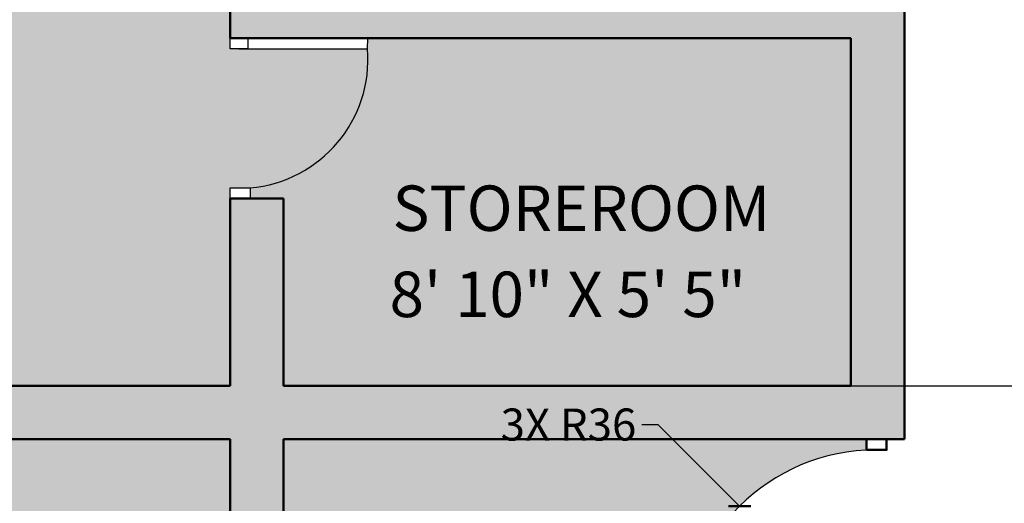
# Model space of a CAD drawing. Units: inches. Extents: x 925 to 2834, y 111 to 1355.
# Tile 18 of 25: x 1553 to 1737, y 882 to 972. Entities that reach past the tile are written whole.
import ezdxf

# ---------------------------------------------------------------- set-up
doc = ezdxf.new("R2010")
doc.units = ezdxf.units.IN
doc.header["$MEASUREMENT"] = 0
for name, color, linetype, lineweight in [('A-ANNO-DIMS', 2, 'Continuous', 18), ('A-AREA-IDEN', 7, 'Continuous', 18), ('A-DOOR', 2, 'Continuous', 25), ('A-FLOR-PATT', 252, 'Continuous', 13), ('A-WALL', 7, 'Continuous', 50)]:
    doc.layers.add(name, color=color, linetype=linetype, lineweight=lineweight)
doc.styles.get("Standard").update_dxf_attribs({"font": 'arial.ttf'})
doc.dimstyles.get("Standard").update_dxf_attribs({"dimtxt": 6, "dimasz": 3, "dimexe": 0.18, "dimexo": 0.0625, "dimgap": 0.09, "dimtad": 0, "dimtih": 1, "dimtoh": 1, "dimdec": 1, "dimzin": 0, "dimdsep": 46, "dimlunit": 3, "dimtxsty": 'Standard', "dimblk": 'ARCHTICK', "dimcen": 0.09, "dimadec": 0, "dimazin": 0, "dimtfac": 1, "dimtdec": 1, "dimtofl": 0, "dimtmove": 0, "dimatfit": 3, "dimfxl": 1, "dimtolj": 1, "dimtzin": 0, "dimarcsym": 0})

# ---------------------------------------------------------------- blocks, each defined once
blk = doc.blocks.new('_ArchTick')
at = {"color": 0, "linetype": 'ByBlock', "const_width": 0.15}
blk.add_lwpolyline([(-0.5, -0.5), (0.5, 0.5)], dxfattribs=at)
blk = doc.blocks.new('*D47')
at = {"layer": 'A-ANNO-DIMS', "color": 0, "lineweight": -2, "transparency": 16777216}
for p, q in [((1708.78, 903.59), (1988.62, 903.59)), ((1988.44, 903.59), (1988.44, 869.23)), ((1988.44, 828.59), (1988.44, 862.95)), ((1708.78, 828.59), (1988.62, 828.59))]:
    blk.add_line(p, q, dxfattribs=at)
at = {"layer": 'Defpoints', "color": 0, "transparency": 16777216}
for p in [(1708.71, 903.59), (1988.44, 903.59), (1708.71, 828.59)]:
    blk.add_point(p, dxfattribs=at)
at = {"layer": 'A-ANNO-DIMS', "color": 0, "lineweight": -2, "transparency": 16777216, "xscale": 3, "yscale": 3, "zscale": 3}
for p, rotation in [((1988.44, 903.59), 90), ((1988.44, 828.59), 270)]:
    blk.add_blockref('_ArchTick', p, dxfattribs=dict(at, rotation=rotation))
at = {"layer": 'A-ANNO-DIMS', "color": 0, "transparency": 16777216, "insert": (1988.44, 866.09), "char_height": 6, "attachment_point": 5}
blk.add_mtext('\\A1;75', dxfattribs=at)
blk = doc.blocks.new('*D48')
at = {"layer": 'A-ANNO-DIMS', "color": 0, "lineweight": -2, "transparency": 16777216}
for p, q in [((1708.78, 975.59), (1988.62, 975.59)), ((1988.44, 975.59), (1988.44, 942.69)), ((1988.44, 903.59), (1988.44, 936.49)), ((1708.78, 903.59), (1988.62, 903.59))]:
    blk.add_line(p, q, dxfattribs=at)
at = {"layer": 'Defpoints', "color": 0, "transparency": 16777216}
for p in [(1708.71, 975.59), (1988.44, 975.59), (1708.71, 903.59)]:
    blk.add_point(p, dxfattribs=at)
at = {"layer": 'A-ANNO-DIMS', "color": 0, "lineweight": -2, "transparency": 16777216, "xscale": 3, "yscale": 3, "zscale": 3}
for p, rotation in [((1988.44, 975.59), 90), ((1988.44, 903.59), 270)]:
    blk.add_blockref('_ArchTick', p, dxfattribs=dict(at, rotation=rotation))
at = {"layer": 'A-ANNO-DIMS', "color": 0, "transparency": 16777216, "insert": (1988.44, 939.59), "char_height": 6, "attachment_point": 5}
blk.add_mtext('\\A1;72', dxfattribs=at)
blk = doc.blocks.new('*D81')
at = {"layer": 'A-ANNO-DIMS', "color": 0, "lineweight": -2, "transparency": 16777216}
for p, q in [((1669.64, 896.32), (1672.64, 896.32)), ((1672.64, 896.32), (1687.92, 881.04)), ((1713.28, 855.59), (1713.46, 855.59)), ((1713.37, 855.5), (1713.37, 855.68))]:
    blk.add_line(p, q, dxfattribs=at)
at = {"layer": 'Defpoints', "color": 0, "transparency": 16777216}
for p in [(1687.92, 881.04), (1713.37, 855.59)]:
    blk.add_point(p, dxfattribs=at)
at = {"layer": 'A-ANNO-DIMS', "color": 0, "lineweight": -2, "transparency": 16777216, "xscale": 3, "yscale": 3, "zscale": 3, "rotation": 315.0000844046568}
blk.add_blockref('_ArchTick', (1687.92, 881.04), dxfattribs=at)
at = {"layer": 'A-ANNO-DIMS', "color": 0, "transparency": 16777216, "insert": (1655.94, 896.32), "char_height": 6, "attachment_point": 5}
blk.add_mtext('\\A1;3X R36', dxfattribs=at)

msp = doc.modelspace()

# ---------------------------------------------------------------- hatches: boundary and pattern name
at = {"layer": 'A-FLOR-PATT', "transparency": 33554605}
h = msp.add_hatch(color=256, dxfattribs=at)
h.dxf.hatch_style = 1
h.paths.add_polyline_path([(1931.688, 1294.5638), (991.7375, 1294.5638), (991.7375, 172.1134), (1931.688, 172.1134)])
h.paths.add_polyline_path([(1910.7128, 1273.5886), (1910.7128, 193.0886), (1012.7128, 193.0886), (1012.7128, 1273.5886)], flags=16)
h.paths.add_polyline_path([(1850.7128, 1213.5886), (1850.7128, 253.0886), (1072.7128, 253.0886), (1072.7128, 1213.5886)], flags=0)
h.paths.add_polyline_path([(1838.7128, 1201.5886), (1838.7128, 265.0886), (1084.7128, 265.0886), (1084.7128, 530.5886), (1084.7128, 1201.5886)], flags=0)
h.paths.add_polyline_path([(1547.6758, 1155.7396), (1547.6758, 1119.115), (1513.0687, 1119.115), (1513.0687, 1155.7396)], flags=0)
h.paths.add_polyline_path([(1600.1067, 1154.9439), (1634.7139, 1154.9439), (1634.7139, 1119.115), (1600.1067, 1119.115)], flags=0)
h.paths.add_polyline_path([(1505.2502, 1144.5358), (1505.2502, 1119.115), (1470.643, 1119.115), (1470.643, 1144.5358)], flags=0)
h.paths.add_polyline_path([(1559.1357, 1141.0962), (1593.7428, 1141.0962), (1593.7428, 1119.115), (1559.1357, 1119.115)], flags=0)
h.paths.add_polyline_path([(1462.8966, 1154.9439), (1462.8966, 1119.115), (1428.2895, 1119.115), (1428.2895, 1154.9439)], flags=0)
h.paths.add_polyline_path([(1642.4603, 1144.5358), (1677.0675, 1144.5358), (1677.0675, 1119.115), (1642.4603, 1119.115)], flags=0)
h.paths.add_polyline_path([(1422.3508, 1141.0962), (1422.3508, 1119.115), (1387.7436, 1119.115), (1387.7436, 1141.0962)], flags=0)
h.paths.add_polyline_path([(1684.8859, 1155.7396), (1719.4931, 1155.7396), (1719.4931, 1119.115), (1684.8859, 1119.115)], flags=0)
h.paths.add_polyline_path([(1718.7128, 1081.5886), (1718.7128, 1050.1249), (1715.7128, 1050.1249), (1715.7128, 1026.1249), (1715.7128, 1002.1249), (1718.7128, 1002.1249), (1730.7128, 1002.1249), (1730.7128, 998.1249), (1730.7128, 990.1249), (1730.7128, 986.1249), (1718.7128, 986.1249), (1718.7128, 893.5886), (1715.3735, 893.5886), (1715.3735, 891.5886), (1713.3735, 891.5886, 0.41421356), (1677.3735, 855.5886), (1713.3735, 855.5886), (1713.3735, 853.5886), (1715.3735, 853.5886), (1715.3735, 851.5886), (1718.7128, 851.5886), (1718.7128, 821.5865), (1734.4655, 821.5865), (1734.3735, 819.5886, -0.41421356), (1712.4415, 793.5886), (1712.4415, 791.5886), (1718.7128, 791.5886), (1718.7128, 717.5886), (1718.7128, 669.5886), (1732.7128, 669.5886), (1732.7128, 665.5886), (1732.7128, 641.5886), (1732.7128, 634.5886), (1732.7128, 610.5886), (1732.7128, 603.5886), (1718.7128, 603.5886), (1718.7128, 385.0886), (1434.2128, 385.0886), (1434.2128, 530.5886), (1410.2128, 530.5886), (1408.2128, 530.5886), (1408.2128, 532.5886, 0.41421356), (1372.2128, 568.5886), (1372.2128, 532.5886), (1370.2128, 532.5886), (1370.2128, 530.5886), (1368.2128, 530.5886), (1282.2128, 530.5886), (1210.2128, 530.5886), (1200.2128, 530.5886), (1200.2128, 542.1915), (1183.2307, 542.1915), (1183.2307, 546.1915), (1200.2128, 546.1915), (1200.2128, 572.1915), (1183.2307, 572.1915), (1183.2307, 576.1915), (1200.2128, 576.1915), (1200.2128, 727.5886), (1210.2128, 727.5886), (1234.2128, 727.5886), (1259.7128, 727.5886), (1259.7128, 775.5886), (1259.7128, 799.5886), (1259.7128, 847.5886), (1259.7128, 993.5872), (1259.7128, 1065.5872), (1259.7128, 1071.5886), (1219.6318, 1071.5886), (1219.6318, 1081.5886), (1084.7128, 1081.5886), (1084.7128, 1119.115), (1256.8974, 1119.115), (1256.8974, 1154.9439), (1291.5046, 1154.9439), (1291.5046, 1119.115), (1256.8974, 1119.115), (1256.6723, 1081.5886), (1293.7128, 1081.5886), (1341.7128, 1081.5886), (1341.7128, 1093.5886), (1347.7128, 1093.5886), (1371.7128, 1093.5886), (1377.7128, 1093.5886), (1377.7128, 1081.5886), (1668.7128, 1081.5886), (1668.7128, 1117.5886), (1675.7128, 1117.5886), (1711.7128, 1117.5886), (1718.7128, 1117.5886)], flags=0)
h.paths.add_polyline_path([(1376.2838, 1155.7396), (1376.2838, 1119.115), (1341.6766, 1119.115), (1341.6766, 1155.7396)], flags=0)
h.paths.add_polyline_path([(1341.7128, 1076.0886), (1293.7128, 1076.0886), (1293.7128, 1071.5886), (1269.7128, 1071.5886), (1269.7128, 1065.5872), (1266.7128, 1065.5872), (1266.7128, 1029.5872), (1265.7128, 1029.5872), (1265.7128, 993.5872), (1269.7128, 993.5872), (1269.7128, 903.5886), (1269.7128, 893.5886), (1269.7128, 847.5886), (1265.2128, 847.5886), (1265.2128, 799.5886), (1269.7128, 799.5886), (1269.7128, 775.5886), (1265.2128, 775.5886), (1265.2128, 727.5886), (1269.7128, 727.5886), (1444.2128, 727.5886), (1444.2128, 717.5886), (1234.2128, 717.5886), (1234.2128, 722.0886), (1210.2128, 722.0886), (1210.2128, 717.5886), (1210.2128, 540.5886), (1210.2128, 536.0886), (1282.2128, 536.0886), (1282.2128, 535.0886), (1210.2128, 535.0886), (1210.2128, 540.5886), (1210.2128, 717.5886), (1210.2128, 723.0886), (1234.2128, 723.0886), (1234.2128, 717.5886), (1444.2128, 717.5886), (1444.2128, 727.5886), (1269.7128, 727.5886), (1264.2128, 727.5886), (1264.2128, 775.5886), (1269.7128, 775.5886), (1269.7128, 799.5886), (1264.2128, 799.5886), (1264.2128, 847.5886), (1269.7128, 847.5886), (1269.7128, 893.5886), (1269.7128, 903.5886), (1269.7128, 993.5872), (1264.7128, 993.5872), (1264.7128, 1029.5872), (1265.7128, 1029.5872), (1265.7128, 1065.5872), (1269.7128, 1065.5872), (1269.7128, 1071.5886), (1293.7128, 1071.5886), (1293.7128, 1077.0886), (1341.7128, 1077.0886)], flags=0)
h.paths.add_polyline_path([(1730.9529, 1141.0962), (1765.5601, 1141.0962), (1765.5601, 1119.115), (1730.9529, 1119.115)], flags=0)
h.paths.add_polyline_path([(1333.8582, 1144.5358), (1333.8582, 1119.115), (1299.251, 1119.115), (1299.251, 1144.5358)], flags=0)
h.paths.add_polyline_path([(1592.7128, 968.5886), (1596.0342, 968.5886), (1602.7128, 968.5886), (1708.7128, 968.5886), (1708.7128, 903.5886), (1602.7128, 903.5886), (1602.7128, 938.5886), (1592.7128, 938.5886), (1592.7128, 903.5886), (1451.7128, 903.5886), (1451.7128, 893.5886), (1511.7128, 893.5886), (1511.7128, 881.5886), (1515.2128, 881.5886), (1518.7128, 881.5886), (1518.7128, 893.5886), (1592.7128, 893.5886), (1592.7128, 799.5886), (1518.7128, 799.5886), (1518.7128, 857.5886), (1511.7128, 857.5886), (1511.7128, 799.5886), (1511.7128, 772.0886), (1521.7128, 772.0886), (1521.7128, 792.5886), (1592.7128, 792.5886), (1592.7128, 727.5886), (1521.7128, 727.5886), (1521.7128, 748.0886), (1511.7128, 748.0886), (1511.7128, 717.5886), (1708.7128, 717.5886), (1714.2128, 717.5886), (1714.2128, 669.5886), (1708.7128, 669.5886), (1708.7128, 641.5886), (1492.2128, 641.5886), (1492.2128, 631.5886), (1621.2128, 631.5886), (1621.2128, 443.0886), (1625.7128, 443.0886), (1625.7128, 503.0886), (1625.7128, 507.5886), (1625.7128, 631.5886), (1708.7128, 631.5886), (1708.7128, 507.5886), (1655.7128, 507.5886), (1655.7128, 503.0886), (1708.7128, 503.0886), (1708.7128, 395.0886), (1625.7128, 395.0886), (1625.7128, 419.0886), (1621.2128, 419.0886), (1621.2128, 395.0886), (1482.2128, 395.0886), (1482.2128, 385.0886), (1434.2128, 385.0886), (1434.2128, 433.0886), (1444.2128, 433.0886), (1444.2128, 631.5886), (1450.2128, 631.5886), (1450.2128, 634.91), (1452.2128, 634.91), (1452.2128, 669.5886), (1454.2128, 669.5886, -0.40021217), (1490.1712, 635.3173), (1492.2128, 635.3173), (1492.2128, 641.5886), (1564.7128, 641.5886), (1564.7128, 677.5886), (1672.7128, 677.5886), (1672.7128, 681.5886), (1564.7128, 681.5886), (1564.7128, 717.5886), (1511.7128, 717.5886), (1511.7128, 748.0886), (1511.7128, 772.0886), (1511.7128, 799.5886), (1511.7128, 857.5886), (1511.8913, 857.5886), (1511.8913, 859.5886), (1515.6201, 859.5886, 0.41421356), (1537.552, 879.5886), (1513.552, 879.5886), (1511.8913, 879.5886), (1511.8913, 881.5886), (1511.7128, 881.5886), (1511.7128, 893.5886), (1451.7128, 893.5886), (1451.7128, 903.5886), (1592.7128, 903.5886), (1592.7128, 938.5886), (1592.7128, 940.5886), (1596.4415, 940.5886, 0.41421356), (1618.3735, 966.5886), (1594.3735, 966.5886), (1592.7128, 966.5886)], flags=0)
h.paths.add_polyline_path([(1377.7128, 903.5886), (1377.7128, 893.5886), (1305.7128, 893.5886), (1305.7128, 903.5886)], flags=0)
h.paths.add_polyline_path([(1708.7128, 821.5886), (1712.0342, 821.5886), (1712.0342, 819.5886), (1710.3735, 819.5886), (1708.7128, 819.5886)], flags=0)
h.paths.add_polyline_path([(1576.7128, 695.1992), (1575.5896, 693.6649), (1575.9687, 694.6994), (1575.4438, 695.1992), (1575.9687, 695.699), (1575.5896, 696.7335)], flags=0)
h.paths.add_polyline_path([(1565.9817, 662.3134), (1565.4568, 661.8136), (1565.8359, 660.7791), (1564.7128, 662.3134), (1565.8359, 663.8477), (1565.4568, 662.8132)], flags=0)
h.paths.add_polyline_path([(1444.2128, 433.0886), (1444.2128, 395.0886), (1482.2128, 395.0886), (1482.2128, 389.0886), (1438.2128, 389.0886), (1438.2128, 391.8608), (1438.2128, 433.0886)], flags=0)
h.paths.add_polyline_path([(1410.2128, 506.5886), (1410.2128, 289.0886), (1108.7128, 289.0886), (1108.7128, 506.5886)], flags=0)
h.paths.add_polyline_path([(1612.3153, 838.3016), (1680.4151, 838.3016), (1680.4151, 851.3131), (1612.3153, 851.3131)], flags=8)
h.paths.add_polyline_path([(1208.3174, 395.0436), (1282.1017, 395.0436), (1282.1017, 408.0552), (1208.3174, 408.0552)], flags=8)
h.paths.add_polyline_path([(1291.8049, 598.7427), (1369.8017, 598.7427), (1369.8017, 611.7542), (1291.8049, 611.7542)], flags=8)
h.paths.add_polyline_path([(1119.679, 917.3022), (1191.0817, 917.3022), (1191.0817, 930.3137), (1119.679, 930.3137)], flags=8)
h.paths.add_polyline_path([(1332.2261, 815.9808), (1410.2258, 815.9808), (1410.2258, 829.001), (1332.2261, 829.001)], flags=8)
h.paths.add_polyline_path([(1390.9013, 955.8158), (1475.4981, 955.8158), (1475.4981, 968.8273), (1390.9013, 968.8273)], flags=8)
h.paths.add_polyline_path([(1620.3436, 998.9325), (1688.4434, 998.9325), (1688.4434, 1011.944), (1620.3436, 1011.944)], flags=8)
h.paths.add_polyline_path([(1620.3436, 914.1039), (1691.7405, 914.1039), (1691.7405, 927.1155), (1620.3436, 927.1155)], flags=8)
h.paths.add_polyline_path([(1521.4542, 816.005), (1589.5569, 816.005), (1589.5569, 829.0253), (1521.4542, 829.0253)], flags=8)
h.paths.add_polyline_path([(1528.524, 740.3497), (1602.3082, 740.3497), (1602.3082, 753.3613), (1528.524, 753.3613)], flags=8)
h.paths.add_polyline_path([(1627.6094, 762.6128), (1702.3091, 762.6128), (1702.3091, 775.6244), (1627.6094, 775.6244)], flags=8)
h.paths.add_polyline_path([(1610.5442, 657.2751), (1684.3284, 657.2751), (1684.3284, 670.2867), (1610.5442, 670.2867)], flags=8)
h.paths.add_polyline_path([(1636.6983, 519.472), (1711.3981, 519.472), (1711.3981, 532.4835), (1636.6983, 532.4835)], flags=8)
h.paths.add_polyline_path([(1616.8577, 424.8539), (1694.8545, 424.8539), (1694.8545, 437.8654), (1616.8577, 437.8654)], flags=8)
h.paths.add_polyline_path([(1506.1456, 460.8838), (1579.9299, 460.8838), (1579.9299, 473.8953), (1506.1456, 473.8953)], flags=8)
h.paths.add_polyline_path([(1624.6119, 784.6011), (1696.9185, 784.6011), (1696.9185, 797.7864), (1624.6119, 797.7864)], flags=8)
h.paths.add_polyline_path([(1606.3732, 854.2194), (1683.3039, 854.2194), (1683.3039, 867.4048), (1606.3732, 867.4048)], flags=8)
h.paths.add_polyline_path([(1127.8008, 940.3581), (1165.1637, 940.3581), (1165.1637, 953.5348), (1127.8008, 953.5348)], flags=8)
h.paths.add_polyline_path([(1620.8657, 1019.4968), (1677.3447, 1019.4968), (1677.3447, 1032.6735), (1620.8657, 1032.6735)], flags=8)
h.paths.add_polyline_path([(1620.8643, 930.1821), (1703.0564, 930.1821), (1703.0564, 943.3675), (1620.8643, 943.3675)], flags=8)
h.paths.add_polyline_path([(1324.5702, 836.8338), (1408.0892, 836.8338), (1408.0892, 850.0191), (1324.5702, 850.0191)], flags=8)
h.paths.add_polyline_path([(1281.6584, 622.8885), (1383.6213, 622.8885), (1383.6213, 636.0739), (1281.6584, 636.0739)], flags=8)
h.paths.add_polyline_path([(1210.6721, 416.7893), (1269.1299, 416.7893), (1269.1299, 429.9747), (1210.6721, 429.9747)], flags=8)
h.paths.add_polyline_path([(1507.8264, 477.4836), (1586.7329, 477.4836), (1586.7329, 490.669), (1507.8264, 490.669)], flags=8)
h.paths.add_polyline_path([(1643.6238, 443.8135), (1696.6696, 443.8135), (1696.6696, 456.5643), (1643.6238, 456.5643)], flags=8)
h.paths.add_polyline_path([(1647.2466, 540.5638), (1693.1825, 540.5638), (1693.1825, 553.7491), (1647.2466, 553.7491)], flags=8)
h.paths.add_polyline_path([(1626.0633, 668.5064), (1673.3174, 668.5064), (1673.3174, 681.6831), (1626.0633, 681.6831)], flags=8)
h.paths.add_polyline_path([(1538.2915, 830.7872), (1567.5942, 830.7872), (1567.5942, 843.5293), (1538.2915, 843.5293)], flags=8)
h.paths.add_polyline_path([(1530.9338, 754.0477), (1559.576, 754.0477), (1559.576, 766.7898), (1530.9338, 766.7898)], flags=8)
h.paths.add_polyline_path([(1351.2461, 979.2309), (1513.8919, 979.2309), (1513.8919, 992.4076), (1351.2461, 992.4076)], flags=8)
at = {"layer": 'A-FLOR-PATT'}
h = msp.add_hatch(color=256, dxfattribs=at)
h.dxf.hatch_style = 1
h.paths.add_polyline_path([(1850.7128, 1213.5886), (1072.7128, 1213.5886), (1072.7128, 253.0886), (1850.7128, 253.0886)])
h.paths.add_polyline_path([(1084.7128, 1201.5886), (1838.7128, 1201.5886), (1838.7128, 265.0886), (1084.7128, 265.0886)], flags=16)
h.paths.add_polyline_path([(1183.2307, 576.1915), (1200.2128, 576.1915), (1200.2128, 727.5886), (1210.2128, 727.5886), (1234.2128, 727.5886), (1259.7128, 727.5886), (1259.7128, 775.5886), (1259.7128, 799.5886), (1259.7128, 847.5886), (1259.7128, 993.5872), (1259.7128, 1065.5872), (1259.7128, 1071.5886), (1219.6318, 1071.5886), (1219.6318, 1081.5886), (1293.7128, 1081.5886), (1341.7128, 1081.5886), (1341.7128, 1093.5886), (1347.7128, 1093.5886), (1347.7128, 1081.5886), (1371.7128, 1081.5886), (1371.7128, 1093.5886), (1377.7128, 1093.5886), (1377.7128, 1081.5886), (1668.7128, 1081.5886), (1668.7128, 1117.5886), (1675.7128, 1117.5886), (1675.7128, 1081.5886), (1711.7128, 1081.5886), (1711.7128, 1117.5886), (1718.7128, 1117.5886), (1718.7128, 1081.5886), (1718.7128, 1050.1249), (1715.7128, 1050.1249), (1715.7128, 1026.1249), (1715.7128, 1002.1249), (1718.7128, 1002.1249), (1730.7128, 1002.1249), (1730.7128, 998.1249), (1730.7128, 990.1249), (1730.7128, 986.1249), (1718.7128, 986.1249), (1718.7128, 893.5886), (1715.3735, 893.5886), (1715.3735, 891.5886), (1713.3735, 891.5886, 0.41421356), (1677.3735, 855.5886), (1713.3735, 855.5886), (1713.3735, 853.5886), (1715.3735, 853.5886), (1715.3735, 851.5886), (1718.7128, 851.5886), (1718.7128, 821.5865), (1734.4655, 821.5865), (1734.3735, 819.5886, -0.41421356), (1712.4415, 793.5886), (1712.4415, 791.5886), (1718.7128, 791.5886), (1718.7128, 717.5886), (1718.7128, 669.5886), (1732.7128, 669.5886), (1732.7128, 665.5886), (1732.7128, 641.5886), (1732.7128, 634.5886), (1732.7128, 610.5886), (1732.7128, 603.5886), (1718.7128, 603.5886), (1718.7128, 385.0886), (1434.2128, 385.0886), (1434.2128, 433.0886), (1434.2128, 530.5886), (1410.2128, 530.5886), (1408.2128, 530.5886), (1408.2128, 532.5886, 0.41421356), (1372.2128, 568.5886), (1372.2128, 532.5886), (1370.2128, 532.5886), (1370.2128, 530.5886), (1368.2128, 530.5886), (1282.2128, 530.5886), (1210.2128, 530.5886), (1200.2128, 530.5886), (1200.2128, 542.1915), (1183.2307, 542.1915), (1183.2307, 546.1915), (1200.2128, 546.1915), (1200.2128, 572.1915), (1183.2307, 572.1915)], flags=0)
h.paths.add_polyline_path([(1210.2128, 717.5886), (1210.2128, 723.0886), (1234.2128, 723.0886), (1234.2128, 717.5886), (1444.2128, 717.5886), (1444.2128, 727.5886), (1269.7128, 727.5886), (1264.2128, 727.5886), (1264.2128, 775.5886), (1269.7128, 775.5886), (1269.7128, 799.5886), (1264.2128, 799.5886), (1264.2128, 847.5886), (1269.7128, 847.5886), (1269.7128, 893.5886), (1269.7128, 903.5886), (1269.7128, 993.5872), (1264.7128, 993.5872), (1264.7128, 1029.5872), (1265.7128, 1029.5872), (1265.7128, 1065.5872), (1269.7128, 1065.5872), (1269.7128, 1071.5886), (1293.7128, 1071.5886), (1293.7128, 1077.0886), (1341.7128, 1077.0886), (1341.7128, 1076.0886), (1293.7128, 1076.0886), (1293.7128, 1071.5886), (1269.7128, 1071.5886), (1269.7128, 1065.5872), (1266.7128, 1065.5872), (1266.7128, 1029.5872), (1265.7128, 1029.5872), (1265.7128, 993.5872), (1269.7128, 993.5872), (1269.7128, 903.5886), (1269.7128, 893.5886), (1269.7128, 847.5886), (1265.2128, 847.5886), (1265.2128, 799.5886), (1269.7128, 799.5886), (1269.7128, 775.5886), (1265.2128, 775.5886), (1265.2128, 727.5886), (1269.7128, 727.5886), (1444.2128, 727.5886), (1444.2128, 717.5886), (1234.2128, 717.5886), (1234.2128, 722.0886), (1210.2128, 722.0886), (1210.2128, 717.5886), (1210.2128, 540.5886), (1210.2128, 536.0886), (1282.2128, 536.0886), (1282.2128, 535.0886), (1210.2128, 535.0886), (1210.2128, 540.5886)], flags=0)
h.paths.add_polyline_path([(1450.2128, 634.91), (1452.2128, 634.91), (1452.2128, 669.5886), (1454.2128, 669.5886, -0.40021217), (1490.1712, 635.3173), (1492.2128, 635.3173), (1492.2128, 641.5886), (1564.7128, 641.5886), (1564.7128, 677.5886), (1672.7128, 677.5886), (1672.7128, 681.5886), (1564.7128, 681.5886), (1564.7128, 717.5886), (1511.7128, 717.5886), (1511.7128, 748.0886), (1511.7128, 772.0886), (1511.7128, 799.5886), (1511.7128, 857.5886), (1511.8913, 857.5886), (1511.8913, 859.5886), (1515.6201, 859.5886, 0.41421356), (1537.552, 879.5886), (1513.552, 879.5886), (1511.8913, 879.5886), (1511.8913, 881.5886), (1511.7128, 881.5886), (1511.7128, 893.5886), (1451.7128, 893.5886), (1451.7128, 903.5886), (1592.7128, 903.5886), (1592.7128, 938.5886), (1592.7128, 940.5886), (1596.4415, 940.5886, 0.41421356), (1618.3735, 966.5886), (1594.3735, 966.5886), (1592.7128, 966.5886), (1592.7128, 968.5886), (1596.0342, 968.5886), (1602.7128, 968.5886), (1708.7128, 968.5886), (1708.7128, 903.5886), (1602.7128, 903.5886), (1602.7128, 938.5886), (1592.7128, 938.5886), (1592.7128, 903.5886), (1451.7128, 903.5886), (1451.7128, 893.5886), (1511.7128, 893.5886), (1511.7128, 881.5886), (1518.7128, 881.5886), (1518.7128, 893.5886), (1592.7128, 893.5886), (1592.7128, 799.5886), (1518.7128, 799.5886), (1518.7128, 857.5886), (1511.7128, 857.5886), (1511.7128, 799.5886), (1511.7128, 772.0886), (1521.7128, 772.0886), (1521.7128, 792.5886), (1592.7128, 792.5886), (1592.7128, 727.5886), (1521.7128, 727.5886), (1521.7128, 748.0886), (1511.7128, 748.0886), (1511.7128, 717.5886), (1708.7128, 717.5886), (1714.2128, 717.5886), (1714.2128, 669.5886), (1708.7128, 669.5886), (1708.7128, 641.5886), (1492.2128, 641.5886), (1492.2128, 631.5886), (1621.2128, 631.5886), (1621.2128, 443.0886), (1625.7128, 443.0886), (1625.7128, 503.0886), (1625.7128, 507.5886), (1625.7128, 631.5886), (1708.7128, 631.5886), (1708.7128, 507.5886), (1655.7128, 507.5886), (1655.7128, 503.0886), (1708.7128, 503.0886), (1708.7128, 395.0886), (1625.7128, 395.0886), (1625.7128, 419.0886), (1621.2128, 419.0886), (1621.2128, 395.0886), (1482.2128, 395.0886), (1482.2128, 389.0886), (1438.2128, 389.0886), (1438.2128, 391.8608), (1438.2128, 433.0886), (1444.2128, 433.0886), (1444.2128, 631.5886), (1450.2128, 631.5886)], flags=0)
h.paths.add_polyline_path([(1444.2128, 433.0886), (1444.2128, 395.0886), (1482.2128, 395.0886), (1482.2128, 391.0886), (1440.2128, 391.0886), (1440.2128, 391.8608), (1440.2128, 433.0886)], flags=0)
h.paths.add_polyline_path([(1305.7128, 893.5886), (1305.7128, 903.5886), (1377.7128, 903.5886), (1377.7128, 893.5886)], flags=0)
h.paths.add_polyline_path([(1564.7128, 662.3134), (1565.8359, 663.8477), (1565.4568, 662.8132), (1565.9817, 662.3134), (1565.4568, 661.8136), (1565.8359, 660.7791)], flags=0)
h.paths.add_polyline_path([(1575.4438, 695.1992), (1575.9687, 695.699), (1575.5896, 696.7335), (1576.7128, 695.1992), (1575.5896, 693.6649), (1575.9687, 694.6994)], flags=0)
h.paths.add_polyline_path([(1708.7128, 821.5886), (1712.0342, 821.5886), (1712.0342, 819.5886), (1710.3735, 819.5886), (1708.7128, 819.5886)], flags=0)
h = msp.add_hatch(color=256, dxfattribs=at)
h.dxf.hatch_style = 1
h.paths.add_polyline_path([(1718.7128, 603.5886), (1708.7128, 603.5886), (1708.7128, 507.5886), (1655.7128, 507.5886), (1655.7128, 503.0886), (1708.7128, 503.0886), (1708.7128, 395.0886), (1625.7128, 395.0886), (1625.7128, 419.0886), (1621.2128, 419.0886), (1621.2128, 395.0886), (1482.2128, 395.0886), (1482.2128, 385.0886), (1718.7128, 385.0886)])
h.paths.add_polyline_path([(1625.7128, 631.5886), (1708.7128, 631.5886), (1708.7128, 603.5886), (1718.7128, 603.5886), (1732.7128, 603.5886), (1732.7128, 610.5886), (1715.7128, 610.5886), (1715.7128, 634.5886), (1732.7128, 634.5886), (1732.7128, 641.5886), (1715.7128, 641.5886), (1715.7128, 665.5886), (1732.7128, 665.5886), (1732.7128, 669.5886), (1708.7128, 669.5886), (1708.7128, 641.5886), (1492.2128, 641.5886), (1492.2128, 631.5886), (1621.2128, 631.5886), (1621.2128, 443.0886), (1625.7128, 443.0886), (1625.7128, 503.0886), (1625.7128, 507.5886)])
h.paths.add_polyline_path([(1718.7128, 851.5886), (1708.7128, 851.5886), (1708.7128, 828.5886), (1602.7128, 828.5886), (1602.7128, 893.5886), (1708.7128, 893.5886), (1718.7128, 893.5886), (1718.7128, 986.1249), (1730.7128, 986.1249), (1730.7128, 990.1249), (1718.7128, 990.1249), (1718.7128, 998.1249), (1730.7128, 998.1249), (1730.7128, 1002.1249), (1718.7128, 1002.1249), (1708.7128, 1002.1249), (1708.7128, 975.5886), (1602.7128, 975.5886), (1602.7128, 1011.5886), (1592.7128, 1011.5886), (1592.7128, 968.5886), (1596.0342, 968.5886), (1602.7128, 968.5886), (1708.7128, 968.5886), (1708.7128, 903.5886), (1602.7128, 903.5886), (1602.7128, 938.5886), (1592.7128, 938.5886), (1592.7128, 903.5886), (1451.7128, 903.5886), (1451.7128, 893.5886), (1511.7128, 893.5886), (1511.7128, 881.5886), (1515.2128, 881.5886), (1518.7128, 881.5886), (1518.7128, 893.5886), (1592.7128, 893.5886), (1592.7128, 799.5886), (1518.7128, 799.5886), (1518.7128, 857.5886), (1511.7128, 857.5886), (1511.7128, 799.5886), (1511.7128, 772.0886), (1521.7128, 772.0886), (1521.7128, 792.5886), (1592.7128, 792.5886), (1592.7128, 727.5886), (1521.7128, 727.5886), (1521.7128, 748.0886), (1511.7128, 748.0886), (1511.7128, 717.5886), (1708.7128, 717.5886), (1718.7128, 717.5886), (1718.7128, 727.5886), (1718.7128, 791.5886), (1708.7128, 791.5886), (1708.7128, 727.5886), (1602.7128, 727.5886), (1602.7128, 821.5886), (1708.7128, 821.5886), (1712.0342, 821.5886), (1718.7128, 821.5886)])
h.paths.add_polyline_path([(1718.7128, 1081.5886), (1718.7128, 1117.5886), (1711.7128, 1117.5886), (1711.7128, 1081.5886), (1675.7128, 1081.5886), (1675.7128, 1117.5886), (1668.7128, 1117.5886), (1668.7128, 1081.5886), (1377.7128, 1081.5886), (1377.7128, 1093.5886), (1371.7128, 1093.5886), (1371.7128, 1081.5886), (1347.7128, 1081.5886), (1347.7128, 1093.5886), (1341.7128, 1093.5886), (1341.7128, 1081.5886), (1341.7128, 1071.5886), (1592.7128, 1071.5886), (1592.7128, 1035.5886), (1602.7128, 1035.5886), (1602.7128, 1071.5886), (1708.7128, 1071.5886), (1708.7128, 1050.1249), (1718.7128, 1050.1249)])
h.paths.add_polyline_path([(1293.7128, 1081.5886), (1219.6318, 1081.5886), (1219.6318, 1071.5886), (1259.7128, 1071.5886), (1259.7128, 1065.5872), (1269.7128, 1065.5872), (1269.7128, 1071.5886), (1293.7128, 1071.5886)])
h.paths.add_polyline_path([(1269.7128, 903.5886), (1269.7128, 993.5872), (1259.7128, 993.5872), (1259.7128, 847.5886), (1269.7128, 847.5886), (1269.7128, 893.5886)])
h.paths.add_polyline_path([(1377.7128, 903.5886), (1305.7128, 903.5886), (1305.7128, 893.5886), (1377.7128, 893.5886)])
h.paths.add_polyline_path([(1444.2128, 727.5886), (1269.7128, 727.5886), (1259.7128, 727.5886), (1234.2128, 727.5886), (1234.2128, 717.5886), (1444.2128, 717.5886)])
h.paths.add_polyline_path([(1269.7128, 799.5886), (1259.7128, 799.5886), (1259.7128, 775.5886), (1269.7128, 775.5886)])
h.paths.add_polyline_path([(1444.2128, 631.5886), (1450.2128, 631.5886), (1450.2128, 634.91), (1450.2128, 641.5886), (1434.2128, 641.5886), (1434.2128, 540.5886), (1410.2128, 540.5886), (1410.2128, 530.5886), (1434.2128, 530.5886), (1434.2128, 433.0886), (1444.2128, 433.0886)])
h.paths.add_polyline_path([(1368.2128, 533.91), (1368.2128, 540.5886), (1282.2128, 540.5886), (1282.2128, 530.5886), (1368.2128, 530.5886)])
h.paths.add_polyline_path([(1210.2128, 717.5886), (1210.2128, 727.5886), (1200.2128, 727.5886), (1200.2128, 576.1915), (1183.2307, 576.1915), (1183.2307, 572.1915), (1200.2128, 572.1915), (1200.2128, 546.1915), (1183.2307, 546.1915), (1183.2307, 542.1915), (1200.2128, 542.1915), (1200.2128, 530.5886), (1210.2128, 530.5886), (1210.2128, 540.5886)])
at = {"layer": 'A-FLOR-PATT', "transparency": 33554605}
h = msp.add_hatch(color=256, dxfattribs=at)
h.dxf.hatch_style = 1
h.paths.add_polyline_path([(1592.7128, 938.5886), (1592.7128, 940.5886), (1596.4415, 940.5886, 0.41421356), (1618.3735, 966.5886), (1594.3735, 966.5886), (1592.7128, 966.5886), (1592.7128, 968.5886), (1592.7128, 1011.5886), (1602.7128, 1011.5886), (1602.7128, 975.5886), (1708.7128, 975.5886), (1708.7128, 1002.1249), (1711.7128, 1002.1249), (1711.7128, 1026.1249), (1711.7128, 1050.1249), (1708.7128, 1050.1249), (1708.7128, 1071.5886), (1602.7128, 1071.5886), (1602.7128, 1035.5886), (1592.7128, 1035.5886), (1592.7128, 1071.5886), (1341.7128, 1071.5886), (1293.7128, 1071.5886), (1269.7128, 1071.5886), (1269.7128, 1065.5872), (1269.7128, 993.5872), (1269.7128, 903.5886), (1269.7128, 893.5886), (1269.7128, 847.5886), (1269.7128, 799.5886), (1269.7128, 775.5886), (1269.7128, 727.5886), (1444.2128, 727.5886), (1444.2128, 717.5886), (1234.2128, 717.5886), (1210.2128, 717.5886), (1210.2128, 540.5886), (1282.2128, 540.5886), (1368.2128, 540.5886), (1368.2128, 533.91), (1370.2128, 533.91), (1370.2128, 568.5886), (1372.2128, 568.5886, -0.40021217), (1408.1712, 534.3173), (1410.2128, 534.3173), (1410.2128, 540.5886), (1434.2128, 540.5886), (1434.2128, 641.5886), (1450.2128, 641.5886), (1450.2128, 634.91), (1452.2128, 634.91), (1452.2128, 669.5886), (1454.2128, 669.5886, -0.40021217), (1490.1712, 635.3173), (1492.2128, 635.3173), (1492.2128, 641.5886), (1564.7128, 641.5886), (1564.7128, 677.5886), (1672.7128, 677.5886), (1672.7128, 681.5886), (1564.7128, 681.5886), (1564.7128, 717.5886), (1511.7128, 717.5886), (1511.7128, 748.0886), (1511.7128, 772.0886), (1511.7128, 799.5886), (1511.7128, 857.5886), (1511.8913, 857.5886), (1511.8913, 859.5886), (1515.6201, 859.5886, 0.41421356), (1537.552, 879.5886), (1513.552, 879.5886), (1511.8913, 879.5886), (1511.8913, 881.5886), (1511.7128, 881.5886), (1511.7128, 893.5886), (1451.7128, 893.5886), (1451.7128, 903.5886), (1592.7128, 903.5886)])
h.paths.add_polyline_path([(1377.7128, 903.5886), (1377.7128, 893.5886), (1305.7128, 893.5886), (1305.7128, 903.5886)], flags=16)
h.paths.add_polyline_path([(1592.7128, 893.5886), (1518.7128, 893.5886), (1518.7128, 881.5865), (1537.6441, 881.5865), (1537.552, 879.5886, -0.41421356), (1515.6201, 859.5886), (1515.6201, 857.5886), (1518.7128, 857.5886), (1518.7128, 799.5886), (1592.7128, 799.5886)], flags=17)
h.paths.add_polyline_path([(1291.8049, 598.7427), (1369.8017, 598.7427), (1369.8017, 611.7542), (1291.8049, 611.7542)], flags=24)
h.paths.add_polyline_path([(1332.2261, 815.9808), (1410.2258, 815.9808), (1410.2258, 829.001), (1332.2261, 829.001)], flags=24)
h.paths.add_polyline_path([(1390.9013, 955.8158), (1475.4981, 955.8158), (1475.4981, 968.8273), (1390.9013, 968.8273)], flags=24)
h.paths.add_polyline_path([(1620.3436, 998.9325), (1688.4434, 998.9325), (1688.4434, 1011.944), (1620.3436, 1011.944)], flags=24)
h.paths.add_polyline_path([(1620.8657, 1019.4968), (1677.3447, 1019.4968), (1677.3447, 1032.6735), (1620.8657, 1032.6735)], flags=24)
h.paths.add_polyline_path([(1324.5702, 836.8338), (1408.0892, 836.8338), (1408.0892, 850.0191), (1324.5702, 850.0191)], flags=24)
h.paths.add_polyline_path([(1281.6584, 622.8885), (1383.6213, 622.8885), (1383.6213, 636.0739), (1281.6584, 636.0739)], flags=24)
h.paths.add_polyline_path([(1626.0633, 668.5064), (1673.3174, 668.5064), (1673.3174, 681.6831), (1626.0633, 681.6831)], flags=25)
h.paths.add_polyline_path([(1351.2461, 979.2309), (1513.8919, 979.2309), (1513.8919, 992.4076), (1351.2461, 992.4076)], flags=24)
h.paths.add_polyline_path([(1521.4542, 816.005), (1589.5569, 816.005), (1589.5569, 829.0253), (1521.4542, 829.0253)], flags=24)
h.paths.add_polyline_path([(1538.2915, 830.7872), (1567.5942, 830.7872), (1567.5942, 843.5293), (1538.2915, 843.5293)], flags=24)
h.paths.add_polyline_path([(1636.6983, 519.472), (1711.3981, 519.472), (1711.3981, 532.4835), (1636.6983, 532.4835)], flags=9)
h.paths.add_polyline_path([(1616.8577, 424.8539), (1694.8545, 424.8539), (1694.8545, 437.8654), (1616.8577, 437.8654)], flags=9)
h.paths.add_polyline_path([(1506.1456, 460.8838), (1579.9299, 460.8838), (1579.9299, 473.8953), (1506.1456, 473.8953)], flags=9)
h.paths.add_polyline_path([(1606.3732, 854.2194), (1683.3039, 854.2194), (1683.3039, 867.4048), (1606.3732, 867.4048)], flags=25)
h.paths.add_polyline_path([(1507.8264, 477.4836), (1586.7329, 477.4836), (1586.7329, 490.669), (1507.8264, 490.669)], flags=9)
h.paths.add_polyline_path([(1643.6238, 443.8135), (1696.6696, 443.8135), (1696.6696, 456.5643), (1643.6238, 456.5643)], flags=9)
h.paths.add_polyline_path([(1647.2466, 540.5638), (1693.1825, 540.5638), (1693.1825, 553.7491), (1647.2466, 553.7491)], flags=25)
h = msp.add_hatch(color=256, dxfattribs=at)
h.dxf.hatch_style = 1
h.paths.add_polyline_path([(1200.2128, 727.5886), (1084.7128, 727.5886), (1084.7128, 530.5886), (1200.2128, 530.5886), (1200.2128, 542.1915), (1183.2307, 542.1915), (1183.2307, 546.1915), (1200.2128, 546.1915), (1200.2128, 572.1915), (1183.2307, 572.1915), (1183.2307, 576.1915), (1200.2128, 576.1915)])
h.paths.add_polyline_path([(1612.3153, 838.3016), (1680.4151, 838.3016), (1680.4151, 851.3131), (1612.3153, 851.3131)], flags=9)
h.paths.add_polyline_path([(1291.8049, 598.7427), (1369.8017, 598.7427), (1369.8017, 611.7542), (1291.8049, 611.7542)], flags=9)
h.paths.add_polyline_path([(1119.679, 917.3022), (1191.0817, 917.3022), (1191.0817, 930.3137), (1119.679, 930.3137)], flags=9)
h.paths.add_polyline_path([(1332.2261, 815.9808), (1410.2258, 815.9808), (1410.2258, 829.001), (1332.2261, 829.001)], flags=9)
h.paths.add_polyline_path([(1390.9013, 955.8158), (1475.4981, 955.8158), (1475.4981, 968.8273), (1390.9013, 968.8273)], flags=9)
h.paths.add_polyline_path([(1620.3436, 998.9325), (1688.4434, 998.9325), (1688.4434, 1011.944), (1620.3436, 1011.944)], flags=9)
h.paths.add_polyline_path([(1620.3436, 914.1039), (1691.7405, 914.1039), (1691.7405, 927.1155), (1620.3436, 927.1155)], flags=9)
h.paths.add_polyline_path([(1521.4542, 816.005), (1589.5569, 816.005), (1589.5569, 829.0253), (1521.4542, 829.0253)], flags=9)
h.paths.add_polyline_path([(1522.4337, 740.3497), (1596.218, 740.3497), (1596.218, 753.3613), (1522.4337, 753.3613)], flags=9)
h.paths.add_polyline_path([(1606.3732, 854.2194), (1683.3039, 854.2194), (1683.3039, 867.4048), (1606.3732, 867.4048)], flags=9)
h.paths.add_polyline_path([(1127.8008, 940.3581), (1165.1637, 940.3581), (1165.1637, 953.5348), (1127.8008, 953.5348)], flags=9)
h.paths.add_polyline_path([(1620.8657, 1019.4968), (1677.3447, 1019.4968), (1677.3447, 1032.6735), (1620.8657, 1032.6735)], flags=9)
h.paths.add_polyline_path([(1620.8643, 930.1821), (1703.0564, 930.1821), (1703.0564, 943.3675), (1620.8643, 943.3675)], flags=9)
h.paths.add_polyline_path([(1324.5702, 836.8338), (1408.0892, 836.8338), (1408.0892, 850.0191), (1324.5702, 850.0191)], flags=9)
h.paths.add_polyline_path([(1281.6584, 622.8885), (1383.6213, 622.8885), (1383.6213, 636.0739), (1281.6584, 636.0739)], flags=9)
h.paths.add_polyline_path([(1626.0633, 668.5064), (1673.3174, 668.5064), (1673.3174, 681.6831), (1626.0633, 681.6831)], flags=9)
h.paths.add_polyline_path([(1538.2915, 830.7872), (1567.5942, 830.7872), (1567.5942, 843.5293), (1538.2915, 843.5293)], flags=9)
h.paths.add_polyline_path([(1351.2461, 979.2309), (1513.8919, 979.2309), (1513.8919, 992.4076), (1351.2461, 992.4076)], flags=9)
h = msp.add_hatch(color=256, dxfattribs=at)
h.dxf.hatch_style = 1
h.paths.add_polyline_path([(1621.2128, 631.5886), (1492.2128, 631.5886), (1490.2128, 631.5886), (1490.2128, 633.5886, 0.41421356), (1454.2128, 669.5886), (1454.2128, 633.5886), (1452.2128, 633.5886), (1452.2128, 631.5886), (1450.2128, 631.5886), (1444.2128, 631.5886), (1444.2128, 395.0886), (1482.2128, 395.0886), (1621.2128, 395.0886), (1621.2128, 419.0886), (1625.7128, 419.0886), (1625.7128, 395.0886), (1708.7128, 395.0886), (1708.7128, 503.0886), (1655.7128, 503.0886), (1655.7128, 507.5886), (1708.7128, 507.5886), (1708.7128, 631.5886), (1625.7128, 631.5886), (1625.7128, 507.5886), (1625.7128, 503.0886), (1625.7128, 443.0886), (1621.2128, 443.0886)])
h.paths.add_polyline_path([(1636.6983, 519.472), (1711.3981, 519.472), (1711.3981, 532.4835), (1636.6983, 532.4835)], flags=9)
h.paths.add_polyline_path([(1616.8577, 424.8539), (1694.8545, 424.8539), (1694.8545, 437.8654), (1616.8577, 437.8654)], flags=24)
h.paths.add_polyline_path([(1506.1456, 460.8838), (1579.9299, 460.8838), (1579.9299, 473.8953), (1506.1456, 473.8953)], flags=24)
h.paths.add_polyline_path([(1507.8264, 477.4836), (1586.7329, 477.4836), (1586.7329, 490.669), (1507.8264, 490.669)], flags=24)
h.paths.add_polyline_path([(1643.6238, 443.8135), (1696.6696, 443.8135), (1696.6696, 456.5643), (1643.6238, 456.5643)], flags=24)
h.paths.add_polyline_path([(1647.2466, 540.5638), (1693.1825, 540.5638), (1693.1825, 553.7491), (1647.2466, 553.7491)], flags=24)
h.paths.add_polyline_path([(1612.3153, 838.3016), (1680.4151, 838.3016), (1680.4151, 851.3131), (1612.3153, 851.3131)], flags=9)
h.paths.add_polyline_path([(1291.8049, 598.7427), (1369.8017, 598.7427), (1369.8017, 611.7542), (1291.8049, 611.7542)], flags=9)
h.paths.add_polyline_path([(1119.679, 917.3022), (1191.0817, 917.3022), (1191.0817, 930.3137), (1119.679, 930.3137)], flags=9)
h.paths.add_polyline_path([(1332.2261, 815.9808), (1410.2258, 815.9808), (1410.2258, 829.001), (1332.2261, 829.001)], flags=9)
h.paths.add_polyline_path([(1390.9013, 955.8158), (1475.4981, 955.8158), (1475.4981, 968.8273), (1390.9013, 968.8273)], flags=9)
h.paths.add_polyline_path([(1620.3436, 998.9325), (1688.4434, 998.9325), (1688.4434, 1011.944), (1620.3436, 1011.944)], flags=9)
h.paths.add_polyline_path([(1620.3436, 914.1039), (1691.7405, 914.1039), (1691.7405, 927.1155), (1620.3436, 927.1155)], flags=9)
h.paths.add_polyline_path([(1521.4542, 816.005), (1589.5569, 816.005), (1589.5569, 829.0253), (1521.4542, 829.0253)], flags=9)
h.paths.add_polyline_path([(1528.524, 740.3497), (1602.3082, 740.3497), (1602.3082, 753.3613), (1528.524, 753.3613)], flags=9)
h.paths.add_polyline_path([(1627.6094, 762.6128), (1702.3091, 762.6128), (1702.3091, 775.6244), (1627.6094, 775.6244)], flags=9)
h.paths.add_polyline_path([(1624.6119, 784.6011), (1696.9185, 784.6011), (1696.9185, 797.7864), (1624.6119, 797.7864)], flags=9)
h.paths.add_polyline_path([(1606.3732, 854.2194), (1683.3039, 854.2194), (1683.3039, 867.4048), (1606.3732, 867.4048)], flags=9)
h.paths.add_polyline_path([(1127.8008, 940.3581), (1165.1637, 940.3581), (1165.1637, 953.5348), (1127.8008, 953.5348)], flags=9)
h.paths.add_polyline_path([(1620.8657, 1019.4968), (1677.3447, 1019.4968), (1677.3447, 1032.6735), (1620.8657, 1032.6735)], flags=9)
h.paths.add_polyline_path([(1620.8643, 930.1821), (1703.0564, 930.1821), (1703.0564, 943.3675), (1620.8643, 943.3675)], flags=9)
h.paths.add_polyline_path([(1324.5702, 836.8338), (1408.0892, 836.8338), (1408.0892, 850.0191), (1324.5702, 850.0191)], flags=9)
h.paths.add_polyline_path([(1281.6584, 622.8885), (1383.6213, 622.8885), (1383.6213, 636.0739), (1281.6584, 636.0739)], flags=9)
h.paths.add_polyline_path([(1626.0633, 668.5064), (1673.3174, 668.5064), (1673.3174, 681.6831), (1626.0633, 681.6831)], flags=9)
h.paths.add_polyline_path([(1538.2915, 830.7872), (1567.5942, 830.7872), (1567.5942, 843.5293), (1538.2915, 843.5293)], flags=9)
h.paths.add_polyline_path([(1530.9338, 754.0477), (1559.576, 754.0477), (1559.576, 766.7898), (1530.9338, 766.7898)], flags=9)
h.paths.add_polyline_path([(1351.2461, 979.2309), (1513.8919, 979.2309), (1513.8919, 992.4076), (1351.2461, 992.4076)], flags=9)
h = msp.add_hatch(color=256, dxfattribs=at)
h.dxf.hatch_style = 1
h.paths.add_polyline_path([(1708.7128, 791.5886), (1708.7128, 793.5886), (1712.4415, 793.5886, 0.41421356), (1734.3735, 819.5886), (1710.3735, 819.5886), (1708.7128, 819.5886), (1708.7128, 821.5886), (1602.7128, 821.5886), (1602.7128, 727.5886), (1708.7128, 727.5886)])
h.paths.add_polyline_path([(1708.7128, 851.5886), (1712.052, 851.5886), (1712.052, 853.5886), (1677.3735, 853.5886), (1677.3735, 855.5886, -0.40021217), (1711.6447, 891.5471), (1711.6447, 893.5886), (1708.7128, 893.5886), (1602.7128, 893.5886), (1602.7128, 828.5886), (1708.7128, 828.5886)])
h.paths.add_polyline_path([(1708.7128, 968.5886), (1618.4656, 968.5886), (1618.3735, 966.5886, -0.41421356), (1596.4415, 940.5886), (1596.4415, 938.5886), (1602.7128, 938.5886), (1602.7128, 903.5886), (1708.7128, 903.5886)])
h.paths.add_polyline_path([(1708.7128, 717.5886), (1672.7128, 717.5886), (1672.7128, 641.5886), (1708.7128, 641.5886)])
h.paths.add_polyline_path([(1588.7128, 717.5886), (1576.7128, 717.5886), (1576.7128, 681.5886), (1588.7128, 681.5886)])
h.paths.add_polyline_path([(1576.7128, 717.5886), (1564.7128, 717.5886), (1564.7128, 695.1992), (1575.4438, 695.1992), (1575.9687, 695.699), (1575.5896, 696.7335), (1576.7128, 695.1992)])
h.paths.add_polyline_path([(1576.7128, 695.1992), (1575.5896, 693.6649), (1575.9687, 694.6994), (1575.4438, 695.1992), (1564.7128, 695.1992), (1564.7128, 681.5886), (1576.7128, 681.5886)])
h.paths.add_polyline_path([(1600.7128, 717.5886), (1588.7128, 717.5886), (1588.7128, 681.5886), (1600.7128, 681.5886)])
h.paths.add_polyline_path([(1612.7128, 717.5886), (1600.7128, 717.5886), (1600.7128, 681.5886), (1612.7128, 681.5886)])
h.paths.add_polyline_path([(1624.7128, 717.5886), (1612.7128, 717.5886), (1612.7128, 681.5886), (1624.7128, 681.5886)])
h.paths.add_polyline_path([(1636.7128, 717.5886), (1624.7128, 717.5886), (1624.7128, 681.5886), (1636.7128, 681.5886)])
h.paths.add_polyline_path([(1648.7128, 717.5886), (1636.7128, 717.5886), (1636.7128, 681.5886), (1648.7128, 681.5886)])
h.paths.add_polyline_path([(1660.7128, 717.5886), (1648.7128, 717.5886), (1648.7128, 681.5886), (1660.7128, 681.5886)])
h.paths.add_polyline_path([(1672.7128, 717.5886), (1660.7128, 717.5886), (1660.7128, 681.5886), (1672.7128, 681.5886)])
h.paths.add_polyline_path([(1576.7128, 662.3134), (1565.9817, 662.3134), (1565.4568, 661.8136), (1565.8359, 660.7791), (1564.7128, 662.3134), (1564.7128, 641.5886), (1576.7128, 641.5886)])
h.paths.add_polyline_path([(1576.7128, 677.5886), (1564.7128, 677.5886), (1564.7128, 662.3134), (1565.8359, 663.8477), (1565.4568, 662.8132), (1565.9817, 662.3134), (1576.7128, 662.3134)])
h.paths.add_polyline_path([(1588.7128, 677.5886), (1576.7128, 677.5886), (1576.7128, 641.5886), (1588.7128, 641.5886)])
h.paths.add_polyline_path([(1600.7128, 677.5886), (1588.7128, 677.5886), (1588.7128, 641.5886), (1600.7128, 641.5886)])
h.paths.add_polyline_path([(1612.7128, 677.5886), (1600.7128, 677.5886), (1600.7128, 641.5886), (1612.7128, 641.5886)])
h.paths.add_polyline_path([(1624.7128, 677.5886), (1612.7128, 677.5886), (1612.7128, 641.5886), (1624.7128, 641.5886)])
h.paths.add_polyline_path([(1636.7128, 677.5886), (1624.7128, 677.5886), (1624.7128, 641.5886), (1636.7128, 641.5886)])
h.paths.add_polyline_path([(1648.7128, 677.5886), (1636.7128, 677.5886), (1636.7128, 641.5886), (1648.7128, 641.5886)])
h.paths.add_polyline_path([(1660.7128, 677.5886), (1648.7128, 677.5886), (1648.7128, 641.5886), (1660.7128, 641.5886)])
h.paths.add_polyline_path([(1672.7128, 677.5886), (1660.7128, 677.5886), (1660.7128, 641.5886), (1672.7128, 641.5886)])
h.paths.add_polyline_path([(1627.6094, 762.6128), (1702.3091, 762.6128), (1702.3091, 775.6244), (1627.6094, 775.6244)], flags=24)
h.paths.add_polyline_path([(1624.6119, 784.6011), (1696.9185, 784.6011), (1696.9185, 797.7864), (1624.6119, 797.7864)], flags=24)
h.paths.add_polyline_path([(1612.3153, 838.3016), (1680.4151, 838.3016), (1680.4151, 851.3131), (1612.3153, 851.3131)], flags=24)
h.paths.add_polyline_path([(1606.3732, 854.2194), (1683.3039, 854.2194), (1683.3039, 867.4048), (1606.3732, 867.4048)], flags=24)
h.paths.add_polyline_path([(1620.3436, 914.1039), (1691.7405, 914.1039), (1691.7405, 927.1155), (1620.3436, 927.1155)], flags=24)
h.paths.add_polyline_path([(1620.8643, 930.1821), (1703.0564, 930.1821), (1703.0564, 943.3675), (1620.8643, 943.3675)], flags=24)
h.paths.add_polyline_path([(1610.5442, 657.2751), (1684.3284, 657.2751), (1684.3284, 670.2867), (1610.5442, 670.2867)], flags=9)
h.paths.add_polyline_path([(1626.0633, 668.5064), (1673.3174, 668.5064), (1673.3174, 681.6831), (1626.0633, 681.6831)], flags=9)

# ---------------------------------------------------------------- linework, layer by layer
at = {"layer": 'A-DOOR'}
for p, q in [((1618.4655, 968.5865), (1596.0342, 968.5865)), ((1618.3735, 966.5886), (1618.4655, 968.5865)), ((1594.3735, 966.5886), (1618.3735, 966.5886))]:
    msp.add_line(p, q, dxfattribs=at)
for points in [[(1596.0342, 968.5886), (1596.0342, 966.5886), (1592.7128, 966.5886), (1592.7128, 968.5886)], [(1596.4415, 940.5886), (1596.4415, 938.5886), (1592.7128, 938.5886), (1592.7128, 940.5886)]]:
    msp.add_lwpolyline(points, close=True, dxfattribs=at)
for centre, radius, start, end in [((1594.4075, 964.5546), 24.0521, 274.851115, 4.851115), ((1713.3735, 855.5886), 36, 90, 180)]:
    msp.add_arc(centre, radius, start, end, dxfattribs=at)
at = {"layer": 'A-WALL'}
for p, q in [((1592.7128, 1011.5886), (1592.7128, 968.5886)), ((1718.7128, 893.5886), (1718.7128, 986.1249)), ((1718.7128, 986.1249), (1718.7128, 893.5886)), ((1602.7128, 968.5886), (1592.7128, 968.5886)), ((1602.7128, 968.5886), (1708.7128, 968.5886)), ((1708.7128, 968.5886), (1708.7128, 962.5886)), ((1708.7128, 968.5886), (1708.7128, 903.5886)), ((1602.7128, 938.5886), (1592.7128, 938.5886)), ((1592.7128, 938.5886), (1592.7128, 903.5886)), ((1602.7128, 938.5886), (1602.7128, 903.5886)), ((1451.7128, 903.5886), (1592.7128, 903.5886)), ((1602.7128, 903.5886), (1708.7128, 903.5886)), ((1518.7128, 893.5886), (1592.7128, 893.5886)), ((1592.7128, 893.5886), (1592.7128, 799.5886)), ((1602.7128, 893.5886), (1708.7128, 893.5886)), ((1602.7128, 893.5886), (1602.7128, 828.5886)), ((1708.7128, 893.5886), (1718.7128, 893.5886)), ((1718.7128, 893.5886), (1715.3735, 893.5886))]:
    msp.add_line(p, q, dxfattribs=at)
msp.add_lwpolyline([(1711.6447, 891.5886), (1711.6447, 893.5886), (1715.3735, 893.5886), (1715.3735, 891.5886)], close=True, dxfattribs=at)

# ---------------------------------------------------------------- texts
at = {"layer": 'A-AREA-IDEN'}
for s, height, p in [('STOREROOM', 8.49473, (1623.0619, 932.5245)), ('8\' 10" X 5\' 5"', 8.494735, (1622.5122, 916.4174))]:
    msp.add_text(s, height=height, dxfattribs=at).set_placement(p)

# ---------------------------------------------------------------- dimensions: what is measured, and where the dimension line sits
at = {"layer": 'A-ANNO-DIMS'}
for base, p1, p2, picture, middle in [((1988.438, 975.5886), (1708.7128, 903.5886), (1708.7128, 975.5886), '*D48', (1988.438, 939.5886)), ((1988.438, 903.5886), (1708.7128, 828.5886), (1708.7128, 903.5886), '*D47', (1988.438, 866.0886))]:
    dim = msp.add_linear_dim(base=base, p1=p1, p2=p2, angle=90, dimstyle='Standard', override={"dimdec": 0, "dimlfac": 1, "dimrnd": 0, "dimzin": 0, "dimdsep": 46, "dimlunit": 2}, dxfattribs=at)
    dim.commit()
    dim.dimension.update_dxf_attribs({"geometry": picture, "text_midpoint": middle})
dim = msp.add_radius_dim(center=(1713.3735, 855.5886), mpoint=(1687.9176, 881.0444), text='3X <>', dimstyle='Standard', override={"dimdec": 0, "dimlfac": 1, "dimrnd": 0, "dimzin": 0, "dimdsep": 46, "dimlunit": 2}, dxfattribs=at)
dim.commit()
dim.dimension.update_dxf_attribs({"geometry": '*D81', "text_midpoint": (1655.9436, 896.3179), "dimtype": 164})

doc.saveas('drawing.dxf')
